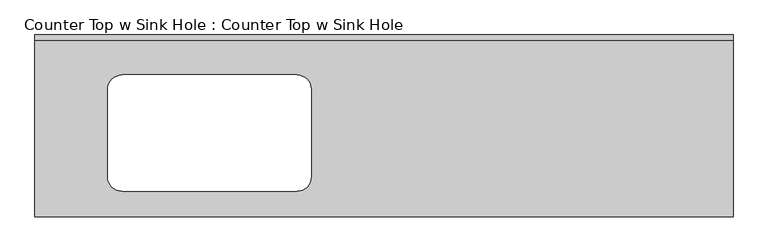
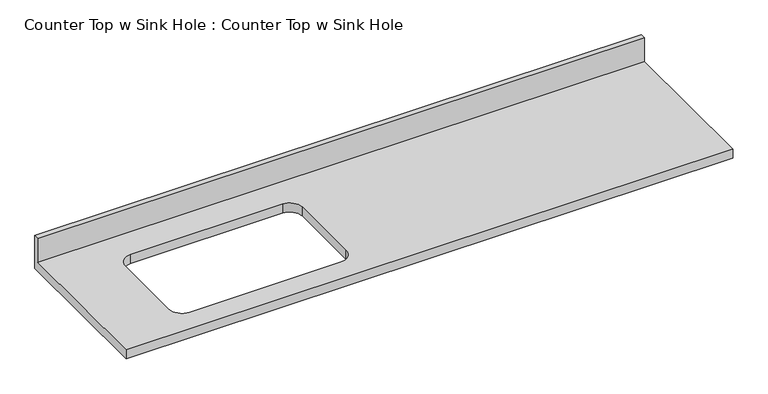
"""IFC4 building model written with IfcOpenShell, lengths in millimetres: furniture geometry, Counter Top w Sink Hole : Counter Top w Sink Hole."""

from ifc_helpers import new_model, si_unit, frame, origin, place, context, project, spatial, polyline, circle_curve, source, transform, mapped, element, save
from ifc_brep_helpers import plane_surface, revolved_surface, advanced_brep


def counter_top_w_sink_hole_counter_top_w_sink_hole_22cae41e(model_context):
    return source(origin(), model_context, "Body", "AdvancedBrep", [
        advanced_brep(
        [(-1200.4622951, -635.0, 914.4), (1237.9377049, -635.0, 914.4), (1237.9377049, -19.05, 914.4), (-1200.4622951, -19.05, 914.4), (-895.6622951, -139.7, 914.4), (-286.0622951, -139.7, 914.4), (-235.2622951, -190.5, 914.4), (-235.2622951, -495.3, 914.4), (-286.0622951, -546.1, 914.4), (-895.6622951, -546.1, 914.4), (-946.4622951, -495.3, 914.4), (-946.4622951, -190.5, 914.4), (1237.9377049, 0.0, 876.3), (1237.9377049, -635.0, 876.3), (-1200.4622951, -635.0, 876.3), (-1200.4622951, 0.0, 876.3), (-286.0622951, -139.7, 876.3), (-895.6622951, -139.7, 876.3), (-946.4622951, -190.5, 876.3), (-946.4622951, -495.3, 876.3), (-895.6622951, -546.1, 876.3), (-286.0622951, -546.1, 876.3), (-235.2622951, -495.3, 876.3), (-235.2622951, -190.5, 876.3), (-1200.4622951, 0.0, 1016.0), (1237.9377049, 0.0, 1016.0), (-1200.4622951, -19.05, 1016.0), (1237.9377049, -19.05, 1016.0)],
        [
            (0, 1),
            (1, 2),
            (2, 3),
            (3, 0),
            (4, 5),
            (5, 6, circle_curve(frame((-286.0622951, -190.5, 914.4), z_axis=(0.0, 0.0, -1.0), x_axis=(1.0, 0.0, 0.0)), 50.8)),
            (6, 7),
            (7, 8, circle_curve(frame((-286.0622951, -495.3, 914.4), z_axis=(0.0, 0.0, -1.0), x_axis=(1.0, 0.0, 0.0)), 50.8)),
            (8, 9),
            (9, 10, circle_curve(frame((-895.6622951, -495.3, 914.4), z_axis=(0.0, 0.0, -1.0), x_axis=(1.0, 0.0, 0.0)), 50.8)),
            (10, 11),
            (11, 4, circle_curve(frame((-895.6622951, -190.5, 914.4), z_axis=(0.0, 0.0, -1.0), x_axis=(1.0, 0.0, 0.0)), 50.8)),
            (12, 13),
            (13, 14),
            (14, 15),
            (15, 12),
            (16, 17),
            (17, 18, circle_curve(frame((-895.6622951, -190.5, 876.3), z_axis=(0.0, 0.0, 1.0), x_axis=(1.0, 0.0, 0.0)), 50.8)),
            (18, 19),
            (19, 20, circle_curve(frame((-895.6622951, -495.3, 876.3), z_axis=(0.0, 0.0, 1.0), x_axis=(1.0, 0.0, 0.0)), 50.8)),
            (20, 21),
            (21, 22, circle_curve(frame((-286.0622951, -495.3, 876.3), z_axis=(0.0, 0.0, 1.0), x_axis=(1.0, 0.0, 0.0)), 50.8)),
            (22, 23),
            (23, 16, circle_curve(frame((-286.0622951, -190.5, 876.3), z_axis=(0.0, 0.0, 1.0), x_axis=(1.0, 0.0, 0.0)), 50.8)),
            (15, 24),
            (24, 25),
            (25, 12),
            (14, 0),
            (3, 26),
            (26, 24),
            (13, 1),
            (25, 27),
            (27, 2),
            (26, 27),
            (4, 17),
            (16, 5),
            (11, 18),
            (10, 19),
            (9, 20),
            (8, 21),
            (7, 22),
            (6, 23),
        ],
        [
            plane_surface(frame((-1200.4622951, 0.0, 914.4), z_axis=(0.0, 0.0, 1.0), x_axis=(-1.0, 0.0, 0.0))),
            plane_surface(frame((-1200.4622951, 0.0, 876.3), z_axis=(0.0, 0.0, -1.0), x_axis=(1.0, 0.0, 0.0))),
            plane_surface(frame((1237.9377049, 0.0, 914.4), z_axis=(0.0, 1.0, 0.0), x_axis=(0.0, 0.0, -1.0))),
            plane_surface(frame((-1200.4622951, 0.0, 914.4), z_axis=(-1.0, 0.0, 0.0), x_axis=(0.0, 0.0, -1.0))),
            plane_surface(frame((-1200.4622951, -635.0, 914.4), z_axis=(0.0, -1.0, 0.0), x_axis=(0.0, 0.0, -1.0))),
            plane_surface(frame((1237.9377049, -635.0, 914.4), z_axis=(1.0, 0.0, 0.0), x_axis=(0.0, 0.0, -1.0))),
            plane_surface(frame((-1200.4622951, 0.0, 1016.0), z_axis=(0.0, 0.0, 1.0), x_axis=(0.0, -1.0, 0.0))),
            plane_surface(frame((-1200.4622951, -19.05, 1016.0), z_axis=(0.0, -1.0, 0.0), x_axis=(0.0, 0.0, -1.0))),
            plane_surface(frame((-286.0622951, -139.7, 914.4), z_axis=(0.0, -1.0, 0.0), x_axis=(0.0, 0.0, -1.0))),
            revolved_surface(polyline([(-844.8622951000001, -190.5, 914.4), (-844.8622951000001, -190.5, 876.3)]), (-895.6622951, -190.5, 876.3), (0.0, 0.0, 1.0)),
            plane_surface(frame((-946.4622951, -190.5, 914.4), z_axis=(1.0, 0.0, 0.0), x_axis=(0.0, 0.0, -1.0))),
            revolved_surface(polyline([(-844.8622951000001, -495.3, 914.4), (-844.8622951000001, -495.3, 876.3)]), (-895.6622951, -495.3, 876.3), (0.0, 0.0, 1.0)),
            plane_surface(frame((-895.6622951, -546.1, 914.4), z_axis=(0.0, 1.0, 0.0), x_axis=(0.0, 0.0, -1.0))),
            revolved_surface(polyline([(-235.26229509999996, -495.3, 914.4), (-235.26229509999996, -495.3, 876.3)]), (-286.0622951, -495.3, 876.3), (0.0, 0.0, 1.0)),
            plane_surface(frame((-235.2622951, -495.3, 914.4), z_axis=(-1.0, 0.0, 0.0), x_axis=(0.0, 0.0, -1.0))),
            revolved_surface(polyline([(-235.26229509999996, -190.5, 914.4), (-235.26229509999996, -190.5, 876.3)]), (-286.0622951, -190.5, 876.3), (0.0, 0.0, 1.0)),
        ],
        [
            (0, [[1, 2, 3, 4], [5, 6, 7, 8, 9, 10, 11, 12]]),
            (1, [[13, 14, 15, 16], [17, 18, 19, 20, 21, 22, 23, 24]]),
            (2, [[-16, 25, 26, 27]]),
            (3, [[-15, 28, -4, 29, 30, -25]]),
            (4, [[-1, -28, -14, 31]]),
            (5, [[-13, -27, 32, 33, -2, -31]]),
            (6, [[-30, 34, -32, -26]]),
            (7, [[-34, -29, -3, -33]]),
            (8, [[35, -17, 36, -5]]),
            (9, [[-35, -12, 37, -18]]),
            (10, [[-37, -11, 38, -19]]),
            (11, [[-38, -10, 39, -20]]),
            (12, [[-39, -9, 40, -21]]),
            (13, [[-40, -8, 41, -22]]),
            (14, [[-41, -7, 42, -23]]),
            (15, [[-36, -24, -42, -6]]),
        ],
    ),
    ])


if __name__ == "__main__":
    model = new_model("IFC4")
    model_context = context("Model", 3, world=origin())
    ifc_project = project(units=[si_unit("LENGTHUNIT", "METRE", prefix="MILLI")], contexts=[model_context])
    site = spatial("IfcSite", under=ifc_project)
    building = spatial("IfcBuilding", under=site)
    placement = place(None, origin())
    counter_top_w_sink_hole_counter_top_w_sink_hole_shape = counter_top_w_sink_hole_counter_top_w_sink_hole_22cae41e(model_context)
    element("IfcFurniture", 1, ObjectType="Counter Top w Sink Hole : Counter Top w Sink Hole", at=placement, inside=building, context=model_context, shape_type="MappedRepresentation", body=[
        mapped(counter_top_w_sink_hole_counter_top_w_sink_hole_shape, transform((0.0, 0.0, 0.0), x_axis=(1.0, 0.0, 0.0), y_axis=(0.0, 1.0, 0.0), z_axis=(0.0, 0.0, 1.0))),
    ])
    save(model, "model.ifc")

# Revit data of these elements
# Type "Counter Top w Sink Hole : Counter Top w Sink Hole"
#   Assembly Code = "C1030400"
#   Counter Thickness = 0' - 1 1/2"
#   Depth = 2' - 1"
#   Height = 3' - 0"
#   Length [instance default] = 8' - 0"
#   Sink Location [instance default] = 2' - 0"
#   Sink Location To Wall [instance default] = 0' - 6"
#   Sink Opening Depth [instance default] = 1' - 3"
#   Sink Opening Width [instance default] = 2' - 3"
#   Counter Top Material = none
#   Default Elevation = 0
# Element 1 (IfcFurniture, "Counter Top w Sink Hole : Counter Top w Sink Hole")
#   Materials on its faces: "Counter Top"
# Materials
#   "Counter Top": class "Wood", colour RGB 226 177 128, transparency 0
